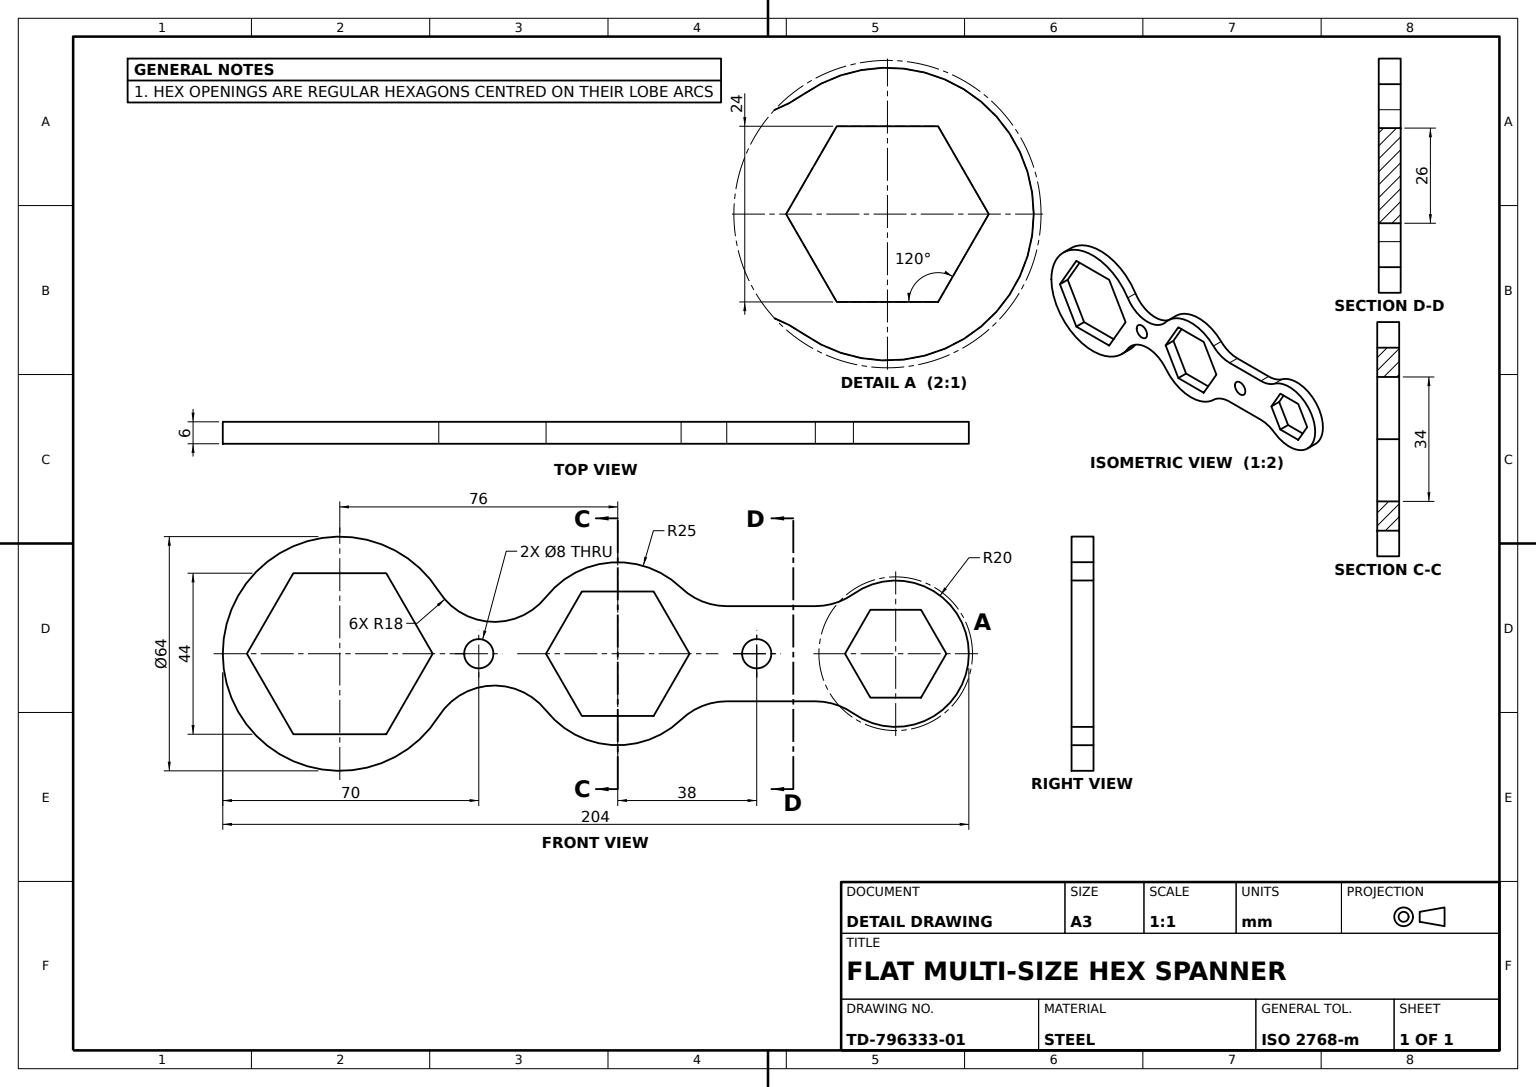
from build123d import *

# Parameters (mm, degrees)
SPANNER_PLATE_6MM_DEPTH        = 6
HEX_OPENINGS_44_34_24_AF_DEPTH = 176.054277297
WEB_HOLES_SKETCH_R             = 4
WEB_HOLES_2X_8_DEPTH           = 176.054277297


with BuildPart() as part:
    # Spanner Outline Sketch → Spanner Plate 6mm (new body)
    with BuildSketch(Plane.XY):
        with BuildLine():
            Line((105.799328852, -13), (130.022739024, -13))
            ThreePointArc((130.022739024, -13), (135.485531832, -13.848968115), (140.433020539, -16.315789474))
            ThreePointArc((140.433020539, -16.315789474), (172, 0), (140.433020539, 16.315789474))
            ThreePointArc((140.433020539, 16.315789474), (135.485531832, 13.848968115), (130.022739024, 13))
            Line((130.022739024, 13), (105.799328852, 13))
            ThreePointArc((105.799328852, 13), (99.075542543, 14.302973388), (93.325191193, 18.023255814))
            ThreePointArc((93.325191193, 18.023255814), (74.306021319, 24.942542698), (56.397031824, 15.515271144))
            ThreePointArc((56.397031824, 15.515271144), (41.324651991, 8.711790831), (27.061052632, 17.079210476))
            ThreePointArc((27.061052632, 17.079210476), (-32, 0), (27.061052632, -17.079210476))
            ThreePointArc((27.061052632, -17.079210476), (41.324651991, -8.711790831), (56.397031824, -15.515271144))
            ThreePointArc((56.397031824, -15.515271144), (74.306021319, -24.942542698), (93.325191193, -18.023255814))
            ThreePointArc((93.325191193, -18.023255814), (99.075542543, -14.302973388), (105.799328852, -13))
        make_face()
    extrude(amount=SPANNER_PLATE_6MM_DEPTH)

    # Hex Openings Sketch → Hex Openings 44-34-24 AF (cut, through all)
    with BuildSketch(Plane.XY.offset(6)):
        Polygon((25.403411844, 0), (12.701705922, 22), (-12.701705922, 22), (-25.403411844, 0), (-12.701705922, -22), (12.701705922, -22), align=None)
        Polygon((95.629909152, 0), (85.814954576, 17), (66.185045424, 17), (56.370090848, 0), (66.185045424, -17), (85.814954576, -17), align=None)
        Polygon((165.856406461, 0), (158.92820323, 12), (145.07179677, 12), (138.143593539, 0), (145.07179677, -12), (158.92820323, -12), align=None)
    extrude(amount=-HEX_OPENINGS_44_34_24_AF_DEPTH, mode=Mode.SUBTRACT)

    # Web Holes Sketch → Web Holes 2xØ8 (cut, through all)
    with BuildSketch(Plane.XY.offset(6)):
        with Locations((38, 0)):
            Circle(WEB_HOLES_SKETCH_R)
        with Locations((114, 0)):
            Circle(WEB_HOLES_SKETCH_R)
    extrude(amount=-WEB_HOLES_2X_8_DEPTH, mode=Mode.SUBTRACT)


solid = part.part
